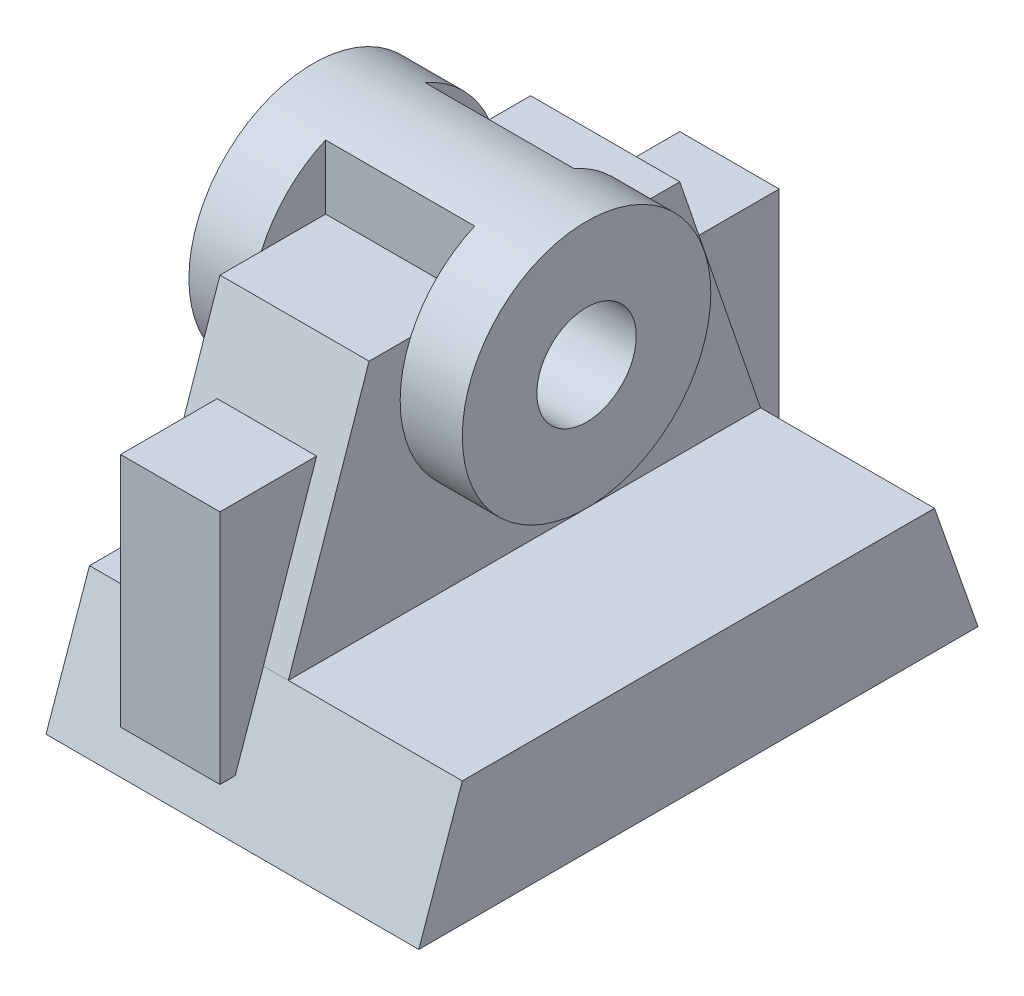
ISO-10303-21;
HEADER;
FILE_DESCRIPTION(('STEP AP214'),'2;1');
FILE_NAME('part.step','',(''),(''),'','','');
FILE_SCHEMA(('AUTOMOTIVE_DESIGN { 1 0 10303 214 1 1 1 1 }'));
ENDSEC;
DATA;
#1=APPLICATION_CONTEXT('core data for automotive mechanical design processes');
#2=APPLICATION_PROTOCOL_DEFINITION('international standard','automotive_design',2000,#1);
#3=PRODUCT_CONTEXT('',#1,'mechanical');
#4=PRODUCT('Part','Part','',(#3));
#5=PRODUCT_RELATED_PRODUCT_CATEGORY('part','',(#4));
#6=PRODUCT_DEFINITION_FORMATION('','',#4);
#7=PRODUCT_DEFINITION_CONTEXT('part definition',#1,'design');
#8=PRODUCT_DEFINITION('design','',#6,#7);
#9=PRODUCT_DEFINITION_SHAPE('','',#8);
#10=(LENGTH_UNIT() NAMED_UNIT(*) SI_UNIT(.MILLI.,.METRE.));
#11=(NAMED_UNIT(*) PLANE_ANGLE_UNIT() SI_UNIT($,.RADIAN.));
#12=(NAMED_UNIT(*) SI_UNIT($,.STERADIAN.) SOLID_ANGLE_UNIT());
#13=UNCERTAINTY_MEASURE_WITH_UNIT(LENGTH_MEASURE(1.E-05),#10,'distance_accuracy_value','');
#14=(GEOMETRIC_REPRESENTATION_CONTEXT(3) GLOBAL_UNCERTAINTY_ASSIGNED_CONTEXT((#13)) GLOBAL_UNIT_ASSIGNED_CONTEXT((#10,
#11,#12)) REPRESENTATION_CONTEXT('',''));
#15=CARTESIAN_POINT('',(0.,0.,0.));
#16=DIRECTION('',(0.,0.,1.));
#17=DIRECTION('',(1.,0.,0.));
#18=AXIS2_PLACEMENT_3D('',#15,#16,#17);
#19=CARTESIAN_POINT('',(-45.,20.,-38.));
#20=DIRECTION('',(0.,-0.330350424728106,0.943858356366018));
#21=DIRECTION('',(0.,-0.943858356366018,-0.330350424728106));
#22=AXIS2_PLACEMENT_3D('',#19,#20,#21);
#23=PLANE('',#22);
#24=DIRECTION('',(0.,-0.943858356366018,-0.330350424728106));
#25=VECTOR('',#24,1.);
#26=CARTESIAN_POINT('',(-2.,20.,-38.));
#27=LINE('',#26,#25);
#28=CARTESIAN_POINT('',(-2.,20.,-38.));
#29=VERTEX_POINT('',#28);
#30=CARTESIAN_POINT('',(-2.,7.,-42.55));
#31=VERTEX_POINT('',#30);
#32=EDGE_CURVE('E233',#29,#31,#27,.T.);
#33=ORIENTED_EDGE('',*,*,#32,.F.);
#34=DIRECTION('',(1.,0.,0.));
#35=VECTOR('',#34,1.);
#36=CARTESIAN_POINT('',(-22.,20.,-38.));
#37=LINE('',#36,#35);
#38=CARTESIAN_POINT('',(2.,20.,-38.));
#39=VERTEX_POINT('',#38);
#40=EDGE_CURVE('E332',#29,#39,#37,.T.);
#41=ORIENTED_EDGE('',*,*,#40,.T.);
#42=DIRECTION('',(1.,0.,0.));
#43=VECTOR('',#42,1.);
#44=CARTESIAN_POINT('',(-45.,20.,-38.));
#45=LINE('',#44,#43);
#46=CARTESIAN_POINT('',(30.,20.,-38.));
#47=VERTEX_POINT('',#46);
#48=EDGE_CURVE('E365',#39,#47,#45,.T.);
#49=ORIENTED_EDGE('',*,*,#48,.T.);
#50=DIRECTION('',(0.,-0.943858356366017,-0.330350424728106));
#51=VECTOR('',#50,1.);
#52=CARTESIAN_POINT('',(30.,20.,-38.));
#53=LINE('',#52,#51);
#54=CARTESIAN_POINT('',(30.,0.,-45.));
#55=VERTEX_POINT('',#54);
#56=EDGE_CURVE('E359',#47,#55,#53,.T.);
#57=ORIENTED_EDGE('',*,*,#56,.T.);
#58=DIRECTION('',(-1.,0.,0.));
#59=VECTOR('',#58,1.);
#60=CARTESIAN_POINT('',(30.,0.,-45.));
#61=LINE('',#60,#59);
#62=CARTESIAN_POINT('',(-30.,0.,-45.));
#63=VERTEX_POINT('',#62);
#64=EDGE_CURVE('E388',#55,#63,#61,.T.);
#65=ORIENTED_EDGE('',*,*,#64,.T.);
#66=DIRECTION('',(0.,-0.943858356366018,-0.330350424728106));
#67=VECTOR('',#66,1.);
#68=CARTESIAN_POINT('',(-30.,17.8173719376392,-38.7639198218263));
#69=LINE('',#68,#67);
#70=CARTESIAN_POINT('',(-30.,20.,-38.));
#71=VERTEX_POINT('',#70);
#72=EDGE_CURVE('E374',#71,#63,#69,.T.);
#73=ORIENTED_EDGE('',*,*,#72,.F.);
#74=CARTESIAN_POINT('',(-22.,20.,-38.));
#75=VERTEX_POINT('',#74);
#76=EDGE_CURVE('E364',#71,#75,#45,.T.);
#77=ORIENTED_EDGE('',*,*,#76,.T.);
#78=CARTESIAN_POINT('',(-18.,20.,-38.));
#79=VERTEX_POINT('',#78);
#80=EDGE_CURVE('E357',#75,#79,#37,.T.);
#81=ORIENTED_EDGE('',*,*,#80,.T.);
#82=DIRECTION('',(0.,0.943858356366018,0.330350424728106));
#83=VECTOR('',#82,1.);
#84=CARTESIAN_POINT('',(-18.,20.,-38.));
#85=LINE('',#84,#83);
#86=CARTESIAN_POINT('',(-18.,7.,-42.55));
#87=VERTEX_POINT('',#86);
#88=EDGE_CURVE('E53',#87,#79,#85,.T.);
#89=ORIENTED_EDGE('',*,*,#88,.F.);
#90=DIRECTION('',(-1.,0.,0.));
#91=VECTOR('',#90,1.);
#92=CARTESIAN_POINT('',(-45.,7.,-42.55));
#93=LINE('',#92,#91);
#94=EDGE_CURVE('E11',#31,#87,#93,.T.);
#95=ORIENTED_EDGE('',*,*,#94,.F.);
#96=EDGE_LOOP('',(#33,#41,#49,#57,#65,#73,#77,#81,#89,#95));
#97=FACE_BOUND('',#96,.T.);
#98=ADVANCED_FACE('F39',(#97),#23,.F.);
#99=CARTESIAN_POINT('',(-22.,20.,-38.));
#100=DIRECTION('',(0.,0.32368767906299,-0.946163984953356));
#101=DIRECTION('',(0.,0.946163984953356,0.32368767906299));
#102=AXIS2_PLACEMENT_3D('',#99,#100,#101);
#103=PLANE('',#102);
#104=ORIENTED_EDGE('',*,*,#40,.F.);
#105=DIRECTION('',(0.,0.946163984953356,0.32368767906299));
#106=VECTOR('',#105,1.);
#107=CARTESIAN_POINT('',(-2.,20.,-38.));
#108=LINE('',#107,#106);
#109=CARTESIAN_POINT('',(-2.,45.,-29.4473684210526));
#110=VERTEX_POINT('',#109);
#111=EDGE_CURVE('E50',#29,#110,#108,.T.);
#112=ORIENTED_EDGE('',*,*,#111,.T.);
#113=DIRECTION('',(-1.,0.,0.));
#114=VECTOR('',#113,1.);
#115=CARTESIAN_POINT('',(-22.,45.,-29.4473684210526));
#116=LINE('',#115,#114);
#117=CARTESIAN_POINT('',(-18.,45.,-29.4473684210526));
#118=VERTEX_POINT('',#117);
#119=EDGE_CURVE('E409',#110,#118,#116,.T.);
#120=ORIENTED_EDGE('',*,*,#119,.T.);
#121=DIRECTION('',(0.,-0.946163984953356,-0.32368767906299));
#122=VECTOR('',#121,1.);
#123=CARTESIAN_POINT('',(-18.,20.,-38.));
#124=LINE('',#123,#122);
#125=EDGE_CURVE('E404',#118,#79,#124,.T.);
#126=ORIENTED_EDGE('',*,*,#125,.T.);
#127=ORIENTED_EDGE('',*,*,#80,.F.);
#128=DIRECTION('',(0.,0.946163984953356,0.32368767906299));
#129=VECTOR('',#128,1.);
#130=CARTESIAN_POINT('',(-22.,20.,-38.));
#131=LINE('',#130,#129);
#132=CARTESIAN_POINT('',(-22.,58.,-25.));
#133=VERTEX_POINT('',#132);
#134=EDGE_CURVE('E314',#75,#133,#131,.T.);
#135=ORIENTED_EDGE('',*,*,#134,.T.);
#136=DIRECTION('',(1.,0.,0.));
#137=VECTOR('',#136,1.);
#138=CARTESIAN_POINT('',(-22.,58.,-25.));
#139=LINE('',#138,#137);
#140=CARTESIAN_POINT('',(2.,58.,-25.));
#141=VERTEX_POINT('',#140);
#142=EDGE_CURVE('E353',#133,#141,#139,.T.);
#143=ORIENTED_EDGE('',*,*,#142,.T.);
#144=DIRECTION('',(0.,0.946163984953356,0.32368767906299));
#145=VECTOR('',#144,1.);
#146=CARTESIAN_POINT('',(2.,20.,-38.));
#147=LINE('',#146,#145);
#148=EDGE_CURVE('E331',#39,#141,#147,.T.);
#149=ORIENTED_EDGE('',*,*,#148,.F.);
#150=EDGE_LOOP('',(#104,#112,#120,#126,#127,#135,#143,#149));
#151=FACE_BOUND('',#150,.T.);
#152=ADVANCED_FACE('F411',(#151),#103,.T.);
#153=CARTESIAN_POINT('',(-32.,50.,0.));
#154=DIRECTION('',(1.,0.,0.));
#155=DIRECTION('',(0.,0.,-1.));
#156=AXIS2_PLACEMENT_3D('',#153,#154,#155);
#157=CYLINDRICAL_SURFACE('',#156,20.);
#158=CARTESIAN_POINT('',(12.,50.,0.));
#159=DIRECTION('',(1.,0.,0.));
#160=DIRECTION('',(0.,0.,-1.));
#161=AXIS2_PLACEMENT_3D('',#158,#159,#160);
#162=CIRCLE('',#161,20.);
#163=CARTESIAN_POINT('',(12.,50.,-20.));
#164=VERTEX_POINT('',#163);
#165=EDGE_CURVE('E302',#164,#164,#162,.T.);
#166=ORIENTED_EDGE('',*,*,#165,.F.);
#167=EDGE_LOOP('',(#166));
#168=FACE_BOUND('',#167,.T.);
#169=CARTESIAN_POINT('',(-32.,50.,0.));
#170=DIRECTION('',(1.,0.,0.));
#171=DIRECTION('',(0.,0.,-1.));
#172=AXIS2_PLACEMENT_3D('',#169,#170,#171);
#173=CIRCLE('',#172,20.);
#174=CARTESIAN_POINT('',(-32.,50.,-20.));
#175=VERTEX_POINT('',#174);
#176=EDGE_CURVE('E306',#175,#175,#173,.T.);
#177=ORIENTED_EDGE('',*,*,#176,.T.);
#178=EDGE_LOOP('',(#177));
#179=FACE_BOUND('',#178,.T.);
#180=DIRECTION('',(1.,0.,0.));
#181=VECTOR('',#180,1.);
#182=CARTESIAN_POINT('',(-22.,68.3303027798234,-8.));
#183=LINE('',#182,#181);
#184=CARTESIAN_POINT('',(-22.,68.3303027798234,-8.));
#185=VERTEX_POINT('',#184);
#186=CARTESIAN_POINT('',(2.,68.3303027798234,-8.));
#187=VERTEX_POINT('',#186);
#188=EDGE_CURVE('E275',#185,#187,#183,.T.);
#189=ORIENTED_EDGE('',*,*,#188,.F.);
#190=CARTESIAN_POINT('',(-22.,50.,0.));
#191=DIRECTION('',(-1.,0.,0.));
#192=DIRECTION('',(0.,0.,1.));
#193=AXIS2_PLACEMENT_3D('',#190,#191,#192);
#194=CIRCLE('',#193,20.);
#195=CARTESIAN_POINT('',(-22.,58.,-18.3303027798234));
#196=VERTEX_POINT('',#195);
#197=EDGE_CURVE('E262',#185,#196,#194,.T.);
#198=ORIENTED_EDGE('',*,*,#197,.T.);
#199=CARTESIAN_POINT('',(-22.,50.,0.));
#200=DIRECTION('',(-1.,0.,0.));
#201=DIRECTION('',(0.,0.,-1.));
#202=AXIS2_PLACEMENT_3D('',#199,#200,#201);
#203=CIRCLE('',#202,20.);
#204=CARTESIAN_POINT('',(-22.,58.,18.3303027798234));
#205=VERTEX_POINT('',#204);
#206=EDGE_CURVE('E321',#196,#205,#203,.T.);
#207=ORIENTED_EDGE('',*,*,#206,.T.);
#208=CARTESIAN_POINT('',(-22.,50.,0.));
#209=DIRECTION('',(1.,0.,0.));
#210=DIRECTION('',(0.,0.,-1.));
#211=AXIS2_PLACEMENT_3D('',#208,#209,#210);
#212=CIRCLE('',#211,20.);
#213=CARTESIAN_POINT('',(-22.,68.3303027798234,8.));
#214=VERTEX_POINT('',#213);
#215=EDGE_CURVE('E283',#214,#205,#212,.T.);
#216=ORIENTED_EDGE('',*,*,#215,.F.);
#217=DIRECTION('',(1.,0.,0.));
#218=VECTOR('',#217,1.);
#219=CARTESIAN_POINT('',(-22.,68.3303027798234,8.));
#220=LINE('',#219,#218);
#221=CARTESIAN_POINT('',(2.,68.3303027798234,8.));
#222=VERTEX_POINT('',#221);
#223=EDGE_CURVE('E301',#214,#222,#220,.T.);
#224=ORIENTED_EDGE('',*,*,#223,.T.);
#225=CARTESIAN_POINT('',(2.,50.,0.));
#226=DIRECTION('',(1.,0.,0.));
#227=DIRECTION('',(0.,0.,-1.));
#228=AXIS2_PLACEMENT_3D('',#225,#226,#227);
#229=CIRCLE('',#228,20.);
#230=CARTESIAN_POINT('',(2.,58.,18.3303027798234));
#231=VERTEX_POINT('',#230);
#232=EDGE_CURVE('E277',#222,#231,#229,.T.);
#233=ORIENTED_EDGE('',*,*,#232,.T.);
#234=CARTESIAN_POINT('',(2.,50.,0.));
#235=DIRECTION('',(-1.,0.,0.));
#236=DIRECTION('',(0.,0.,-1.));
#237=AXIS2_PLACEMENT_3D('',#234,#235,#236);
#238=CIRCLE('',#237,20.);
#239=CARTESIAN_POINT('',(2.,58.,-18.3303027798234));
#240=VERTEX_POINT('',#239);
#241=EDGE_CURVE('E338',#240,#231,#238,.T.);
#242=ORIENTED_EDGE('',*,*,#241,.F.);
#243=CARTESIAN_POINT('',(2.,50.,0.));
#244=DIRECTION('',(-1.,0.,0.));
#245=DIRECTION('',(0.,0.,1.));
#246=AXIS2_PLACEMENT_3D('',#243,#244,#245);
#247=CIRCLE('',#246,20.);
#248=EDGE_CURVE('E263',#187,#240,#247,.T.);
#249=ORIENTED_EDGE('',*,*,#248,.F.);
#250=EDGE_LOOP('',(#189,#198,#207,#216,#224,#233,#242,#249));
#251=FACE_BOUND('',#250,.T.);
#252=ADVANCED_FACE('F487',(#168,#179,#251),#157,.T.);
#253=CARTESIAN_POINT('',(0.,20.,0.));
#254=DIRECTION('',(0.,1.,0.));
#255=DIRECTION('',(0.,0.,1.));
#256=AXIS2_PLACEMENT_3D('',#253,#254,#255);
#257=PLANE('',#256);
#258=DIRECTION('',(1.,0.,0.));
#259=VECTOR('',#258,1.);
#260=CARTESIAN_POINT('',(-45.,20.,38.));
#261=LINE('',#260,#259);
#262=CARTESIAN_POINT('',(-30.,20.,38.));
#263=VERTEX_POINT('',#262);
#264=CARTESIAN_POINT('',(-22.,20.,38.));
#265=VERTEX_POINT('',#264);
#266=EDGE_CURVE('E361',#263,#265,#261,.T.);
#267=ORIENTED_EDGE('',*,*,#266,.T.);
#268=DIRECTION('',(0.,0.,-1.));
#269=VECTOR('',#268,1.);
#270=CARTESIAN_POINT('',(-22.,20.,38.));
#271=LINE('',#270,#269);
#272=EDGE_CURVE('E315',#265,#75,#271,.T.);
#273=ORIENTED_EDGE('',*,*,#272,.T.);
#274=ORIENTED_EDGE('',*,*,#76,.F.);
#275=DIRECTION('',(0.,0.,1.));
#276=VECTOR('',#275,1.);
#277=CARTESIAN_POINT('',(-30.,20.,-45.));
#278=LINE('',#277,#276);
#279=EDGE_CURVE('E385',#71,#263,#278,.T.);
#280=ORIENTED_EDGE('',*,*,#279,.T.);
#281=EDGE_LOOP('',(#267,#273,#274,#280));
#282=FACE_BOUND('',#281,.T.);
#283=ADVANCED_FACE('F423',(#282),#257,.T.);
#284=CARTESIAN_POINT('',(30.,20.,0.));
#285=DIRECTION('',(-1.,0.,0.));
#286=DIRECTION('',(0.,0.,1.));
#287=AXIS2_PLACEMENT_3D('',#284,#285,#286);
#288=PLANE('',#287);
#289=DIRECTION('',(0.,0.,-1.));
#290=VECTOR('',#289,1.);
#291=CARTESIAN_POINT('',(30.,0.,0.));
#292=LINE('',#291,#290);
#293=CARTESIAN_POINT('',(30.,0.,45.));
#294=VERTEX_POINT('',#293);
#295=EDGE_CURVE('E377',#294,#55,#292,.T.);
#296=ORIENTED_EDGE('',*,*,#295,.T.);
#297=ORIENTED_EDGE('',*,*,#56,.F.);
#298=DIRECTION('',(0.,0.,-1.));
#299=VECTOR('',#298,1.);
#300=CARTESIAN_POINT('',(30.,20.,45.));
#301=LINE('',#300,#299);
#302=CARTESIAN_POINT('',(30.,20.,38.));
#303=VERTEX_POINT('',#302);
#304=EDGE_CURVE('E378',#303,#47,#301,.T.);
#305=ORIENTED_EDGE('',*,*,#304,.F.);
#306=DIRECTION('',(0.,0.943858356366017,-0.330350424728106));
#307=VECTOR('',#306,1.);
#308=CARTESIAN_POINT('',(30.,20.,38.));
#309=LINE('',#308,#307);
#310=EDGE_CURVE('E352',#294,#303,#309,.T.);
#311=ORIENTED_EDGE('',*,*,#310,.F.);
#312=EDGE_LOOP('',(#296,#297,#305,#311));
#313=FACE_BOUND('',#312,.T.);
#314=ADVANCED_FACE('F41',(#313),#288,.F.);
#315=CARTESIAN_POINT('',(-30.,20.,-45.));
#316=DIRECTION('',(1.,0.,0.));
#317=DIRECTION('',(0.,0.,-1.));
#318=AXIS2_PLACEMENT_3D('',#315,#316,#317);
#319=PLANE('',#318);
#320=ORIENTED_EDGE('',*,*,#279,.F.);
#321=ORIENTED_EDGE('',*,*,#72,.T.);
#322=DIRECTION('',(0.,0.,1.));
#323=VECTOR('',#322,1.);
#324=CARTESIAN_POINT('',(-30.,0.,-45.));
#325=LINE('',#324,#323);
#326=CARTESIAN_POINT('',(-30.,0.,45.));
#327=VERTEX_POINT('',#326);
#328=EDGE_CURVE('E391',#63,#327,#325,.T.);
#329=ORIENTED_EDGE('',*,*,#328,.T.);
#330=DIRECTION('',(0.,0.943858356366017,-0.330350424728106));
#331=VECTOR('',#330,1.);
#332=CARTESIAN_POINT('',(-30.,45.8797327394209,28.9420935412027));
#333=LINE('',#332,#331);
#334=EDGE_CURVE('E370',#327,#263,#333,.T.);
#335=ORIENTED_EDGE('',*,*,#334,.T.);
#336=EDGE_LOOP('',(#320,#321,#329,#335));
#337=FACE_BOUND('',#336,.T.);
#338=ADVANCED_FACE('F471',(#337),#319,.F.);
#339=DIRECTION('',(0.,0.,-1.));
#340=VECTOR('',#339,1.);
#341=CARTESIAN_POINT('',(2.,20.,-38.));
#342=LINE('',#341,#340);
#343=CARTESIAN_POINT('',(2.,20.,38.));
#344=VERTEX_POINT('',#343);
#345=EDGE_CURVE('E307',#344,#39,#342,.T.);
#346=ORIENTED_EDGE('',*,*,#345,.F.);
#347=EDGE_CURVE('E369',#344,#303,#261,.T.);
#348=ORIENTED_EDGE('',*,*,#347,.T.);
#349=ORIENTED_EDGE('',*,*,#304,.T.);
#350=ORIENTED_EDGE('',*,*,#48,.F.);
#351=EDGE_LOOP('',(#346,#348,#349,#350));
#352=FACE_BOUND('',#351,.T.);
#353=ADVANCED_FACE('F459',(#352),#257,.T.);
#354=CARTESIAN_POINT('',(0.,0.,0.));
#355=DIRECTION('',(0.,1.,0.));
#356=DIRECTION('',(0.,0.,1.));
#357=AXIS2_PLACEMENT_3D('',#354,#355,#356);
#358=PLANE('',#357);
#359=ORIENTED_EDGE('',*,*,#295,.F.);
#360=DIRECTION('',(1.,0.,0.));
#361=VECTOR('',#360,1.);
#362=CARTESIAN_POINT('',(-30.,0.,45.));
#363=LINE('',#362,#361);
#364=EDGE_CURVE('E384',#327,#294,#363,.T.);
#365=ORIENTED_EDGE('',*,*,#364,.F.);
#366=ORIENTED_EDGE('',*,*,#328,.F.);
#367=ORIENTED_EDGE('',*,*,#64,.F.);
#368=EDGE_LOOP('',(#359,#365,#366,#367));
#369=FACE_BOUND('',#368,.T.);
#370=ADVANCED_FACE('F468',(#369),#358,.F.);
#371=CARTESIAN_POINT('',(-45.,20.,38.));
#372=DIRECTION('',(0.,-0.330350424728106,-0.943858356366017));
#373=DIRECTION('',(0.,0.943858356366017,-0.330350424728106));
#374=AXIS2_PLACEMENT_3D('',#371,#372,#373);
#375=PLANE('',#374);
#376=DIRECTION('',(-1.,0.,0.));
#377=VECTOR('',#376,1.);
#378=CARTESIAN_POINT('',(-45.,7.,42.55));
#379=LINE('',#378,#377);
#380=CARTESIAN_POINT('',(-2.,7.,42.55));
#381=VERTEX_POINT('',#380);
#382=CARTESIAN_POINT('',(-18.,7.,42.55));
#383=VERTEX_POINT('',#382);
#384=EDGE_CURVE('E61',#381,#383,#379,.T.);
#385=ORIENTED_EDGE('',*,*,#384,.T.);
#386=DIRECTION('',(0.,0.943858356366017,-0.330350424728106));
#387=VECTOR('',#386,1.);
#388=CARTESIAN_POINT('',(-18.,20.,38.));
#389=LINE('',#388,#387);
#390=CARTESIAN_POINT('',(-18.,20.,38.));
#391=VERTEX_POINT('',#390);
#392=EDGE_CURVE('E253',#383,#391,#389,.T.);
#393=ORIENTED_EDGE('',*,*,#392,.T.);
#394=DIRECTION('',(1.,0.,0.));
#395=VECTOR('',#394,1.);
#396=CARTESIAN_POINT('',(-22.,20.,38.));
#397=LINE('',#396,#395);
#398=EDGE_CURVE('E348',#265,#391,#397,.T.);
#399=ORIENTED_EDGE('',*,*,#398,.F.);
#400=ORIENTED_EDGE('',*,*,#266,.F.);
#401=ORIENTED_EDGE('',*,*,#334,.F.);
#402=ORIENTED_EDGE('',*,*,#364,.T.);
#403=ORIENTED_EDGE('',*,*,#310,.T.);
#404=ORIENTED_EDGE('',*,*,#347,.F.);
#405=CARTESIAN_POINT('',(-2.,20.,38.));
#406=VERTEX_POINT('',#405);
#407=EDGE_CURVE('E355',#406,#344,#397,.T.);
#408=ORIENTED_EDGE('',*,*,#407,.F.);
#409=DIRECTION('',(0.,-0.943858356366017,0.330350424728106));
#410=VECTOR('',#409,1.);
#411=CARTESIAN_POINT('',(-2.,20.,38.));
#412=LINE('',#411,#410);
#413=EDGE_CURVE('E247',#406,#381,#412,.T.);
#414=ORIENTED_EDGE('',*,*,#413,.T.);
#415=EDGE_LOOP('',(#385,#393,#399,#400,#401,#402,#403,#404,#408,#414));
#416=FACE_BOUND('',#415,.T.);
#417=ADVANCED_FACE('F435',(#416),#375,.F.);
#418=CARTESIAN_POINT('',(-22.,20.,38.));
#419=DIRECTION('',(0.,0.32368767906299,0.946163984953356));
#420=DIRECTION('',(0.,-0.946163984953356,0.32368767906299));
#421=AXIS2_PLACEMENT_3D('',#418,#419,#420);
#422=PLANE('',#421);
#423=DIRECTION('',(0.,-0.946163984953356,0.32368767906299));
#424=VECTOR('',#423,1.);
#425=CARTESIAN_POINT('',(-18.,20.,38.));
#426=LINE('',#425,#424);
#427=CARTESIAN_POINT('',(-18.,45.,29.4473684210526));
#428=VERTEX_POINT('',#427);
#429=EDGE_CURVE('E398',#428,#391,#426,.T.);
#430=ORIENTED_EDGE('',*,*,#429,.F.);
#431=DIRECTION('',(-1.,0.,0.));
#432=VECTOR('',#431,1.);
#433=CARTESIAN_POINT('',(-22.,45.,29.4473684210526));
#434=LINE('',#433,#432);
#435=CARTESIAN_POINT('',(-2.,45.,29.4473684210526));
#436=VERTEX_POINT('',#435);
#437=EDGE_CURVE('E400',#436,#428,#434,.T.);
#438=ORIENTED_EDGE('',*,*,#437,.F.);
#439=DIRECTION('',(0.,0.946163984953356,-0.32368767906299));
#440=VECTOR('',#439,1.);
#441=CARTESIAN_POINT('',(-2.,20.,38.));
#442=LINE('',#441,#440);
#443=EDGE_CURVE('E389',#406,#436,#442,.T.);
#444=ORIENTED_EDGE('',*,*,#443,.F.);
#445=ORIENTED_EDGE('',*,*,#407,.T.);
#446=DIRECTION('',(0.,-0.946163984953356,0.32368767906299));
#447=VECTOR('',#446,1.);
#448=CARTESIAN_POINT('',(2.,20.,38.));
#449=LINE('',#448,#447);
#450=CARTESIAN_POINT('',(2.,58.,25.));
#451=VERTEX_POINT('',#450);
#452=EDGE_CURVE('E317',#451,#344,#449,.T.);
#453=ORIENTED_EDGE('',*,*,#452,.F.);
#454=DIRECTION('',(1.,0.,0.));
#455=VECTOR('',#454,1.);
#456=CARTESIAN_POINT('',(-22.,58.,25.));
#457=LINE('',#456,#455);
#458=CARTESIAN_POINT('',(-22.,58.,25.));
#459=VERTEX_POINT('',#458);
#460=EDGE_CURVE('E354',#459,#451,#457,.T.);
#461=ORIENTED_EDGE('',*,*,#460,.F.);
#462=DIRECTION('',(0.,-0.946163984953356,0.32368767906299));
#463=VECTOR('',#462,1.);
#464=CARTESIAN_POINT('',(-22.,20.,38.));
#465=LINE('',#464,#463);
#466=EDGE_CURVE('E328',#459,#265,#465,.T.);
#467=ORIENTED_EDGE('',*,*,#466,.T.);
#468=ORIENTED_EDGE('',*,*,#398,.T.);
#469=EDGE_LOOP('',(#430,#438,#444,#445,#453,#461,#467,#468));
#470=FACE_BOUND('',#469,.T.);
#471=ADVANCED_FACE('F427',(#470),#422,.T.);
#472=CARTESIAN_POINT('',(-22.,58.,25.));
#473=DIRECTION('',(0.,1.,0.));
#474=DIRECTION('',(0.,0.,1.));
#475=AXIS2_PLACEMENT_3D('',#472,#473,#474);
#476=PLANE('',#475);
#477=DIRECTION('',(0.,0.,1.));
#478=VECTOR('',#477,1.);
#479=CARTESIAN_POINT('',(2.,58.,25.));
#480=LINE('',#479,#478);
#481=EDGE_CURVE('E345',#231,#451,#480,.T.);
#482=ORIENTED_EDGE('',*,*,#481,.F.);
#483=DIRECTION('',(0.,0.,-1.));
#484=VECTOR('',#483,1.);
#485=CARTESIAN_POINT('',(2.,58.,18.3303027798234));
#486=LINE('',#485,#484);
#487=CARTESIAN_POINT('',(2.,58.,8.));
#488=VERTEX_POINT('',#487);
#489=EDGE_CURVE('E298',#231,#488,#486,.T.);
#490=ORIENTED_EDGE('',*,*,#489,.T.);
#491=DIRECTION('',(1.,0.,0.));
#492=VECTOR('',#491,1.);
#493=CARTESIAN_POINT('',(-22.,58.,8.));
#494=LINE('',#493,#492);
#495=CARTESIAN_POINT('',(-22.,58.,8.));
#496=VERTEX_POINT('',#495);
#497=EDGE_CURVE('E291',#496,#488,#494,.T.);
#498=ORIENTED_EDGE('',*,*,#497,.F.);
#499=DIRECTION('',(0.,0.,-1.));
#500=VECTOR('',#499,1.);
#501=CARTESIAN_POINT('',(-22.,58.,18.3303027798234));
#502=LINE('',#501,#500);
#503=EDGE_CURVE('E287',#205,#496,#502,.T.);
#504=ORIENTED_EDGE('',*,*,#503,.F.);
#505=DIRECTION('',(0.,0.,1.));
#506=VECTOR('',#505,1.);
#507=CARTESIAN_POINT('',(-22.,58.,25.));
#508=LINE('',#507,#506);
#509=EDGE_CURVE('E322',#205,#459,#508,.T.);
#510=ORIENTED_EDGE('',*,*,#509,.T.);
#511=ORIENTED_EDGE('',*,*,#460,.T.);
#512=EDGE_LOOP('',(#482,#490,#498,#504,#510,#511));
#513=FACE_BOUND('',#512,.T.);
#514=ADVANCED_FACE('F512',(#513),#476,.T.);
#515=CARTESIAN_POINT('',(-22.,58.,-25.));
#516=DIRECTION('',(0.,1.,0.));
#517=DIRECTION('',(0.,0.,1.));
#518=AXIS2_PLACEMENT_3D('',#515,#516,#517);
#519=PLANE('',#518);
#520=DIRECTION('',(0.,0.,1.));
#521=VECTOR('',#520,1.);
#522=CARTESIAN_POINT('',(2.,58.,-25.));
#523=LINE('',#522,#521);
#524=EDGE_CURVE('E340',#141,#240,#523,.T.);
#525=ORIENTED_EDGE('',*,*,#524,.F.);
#526=ORIENTED_EDGE('',*,*,#142,.F.);
#527=DIRECTION('',(0.,0.,1.));
#528=VECTOR('',#527,1.);
#529=CARTESIAN_POINT('',(-22.,58.,-25.));
#530=LINE('',#529,#528);
#531=EDGE_CURVE('E316',#133,#196,#530,.T.);
#532=ORIENTED_EDGE('',*,*,#531,.T.);
#533=DIRECTION('',(0.,0.,1.));
#534=VECTOR('',#533,1.);
#535=CARTESIAN_POINT('',(-22.,58.,-18.3303027798234));
#536=LINE('',#535,#534);
#537=CARTESIAN_POINT('',(-22.,58.,-8.));
#538=VERTEX_POINT('',#537);
#539=EDGE_CURVE('E268',#196,#538,#536,.T.);
#540=ORIENTED_EDGE('',*,*,#539,.T.);
#541=DIRECTION('',(1.,0.,0.));
#542=VECTOR('',#541,1.);
#543=CARTESIAN_POINT('',(-22.,58.,-8.));
#544=LINE('',#543,#542);
#545=CARTESIAN_POINT('',(2.,58.,-8.));
#546=VERTEX_POINT('',#545);
#547=EDGE_CURVE('E276',#538,#546,#544,.T.);
#548=ORIENTED_EDGE('',*,*,#547,.T.);
#549=DIRECTION('',(0.,0.,1.));
#550=VECTOR('',#549,1.);
#551=CARTESIAN_POINT('',(2.,58.,-18.3303027798234));
#552=LINE('',#551,#550);
#553=EDGE_CURVE('E269',#240,#546,#552,.T.);
#554=ORIENTED_EDGE('',*,*,#553,.F.);
#555=EDGE_LOOP('',(#525,#526,#532,#540,#548,#554));
#556=FACE_BOUND('',#555,.T.);
#557=ADVANCED_FACE('F513',(#556),#519,.T.);
#558=CARTESIAN_POINT('',(-22.,50.,0.));
#559=DIRECTION('',(1.,0.,0.));
#560=DIRECTION('',(0.,0.,-1.));
#561=AXIS2_PLACEMENT_3D('',#558,#559,#560);
#562=PLANE('',#561);
#563=ORIENTED_EDGE('',*,*,#272,.F.);
#564=ORIENTED_EDGE('',*,*,#466,.F.);
#565=ORIENTED_EDGE('',*,*,#509,.F.);
#566=ORIENTED_EDGE('',*,*,#206,.F.);
#567=ORIENTED_EDGE('',*,*,#531,.F.);
#568=ORIENTED_EDGE('',*,*,#134,.F.);
#569=EDGE_LOOP('',(#563,#564,#565,#566,#567,#568));
#570=FACE_BOUND('',#569,.T.);
#571=ADVANCED_FACE('F424',(#570),#562,.F.);
#572=CARTESIAN_POINT('',(2.,50.,0.));
#573=DIRECTION('',(1.,0.,0.));
#574=DIRECTION('',(0.,0.,-1.));
#575=AXIS2_PLACEMENT_3D('',#572,#573,#574);
#576=PLANE('',#575);
#577=ORIENTED_EDGE('',*,*,#452,.T.);
#578=ORIENTED_EDGE('',*,*,#345,.T.);
#579=ORIENTED_EDGE('',*,*,#148,.T.);
#580=ORIENTED_EDGE('',*,*,#524,.T.);
#581=ORIENTED_EDGE('',*,*,#241,.T.);
#582=ORIENTED_EDGE('',*,*,#481,.T.);
#583=EDGE_LOOP('',(#577,#578,#579,#580,#581,#582));
#584=FACE_BOUND('',#583,.T.);
#585=ADVANCED_FACE('F456',(#584),#576,.T.);
#586=CARTESIAN_POINT('',(-32.,50.,0.));
#587=DIRECTION('',(1.,0.,0.));
#588=DIRECTION('',(0.,0.,-1.));
#589=AXIS2_PLACEMENT_3D('',#586,#587,#588);
#590=PLANE('',#589);
#591=CARTESIAN_POINT('',(-32.,50.,0.));
#592=DIRECTION('',(1.,0.,0.));
#593=DIRECTION('',(0.,0.,-1.));
#594=AXIS2_PLACEMENT_3D('',#591,#592,#593);
#595=CIRCLE('',#594,8.);
#596=CARTESIAN_POINT('',(-32.,50.,-8.));
#597=VERTEX_POINT('',#596);
#598=EDGE_CURVE('E257',#597,#597,#595,.T.);
#599=ORIENTED_EDGE('',*,*,#598,.T.);
#600=EDGE_LOOP('',(#599));
#601=FACE_BOUND('',#600,.T.);
#602=ORIENTED_EDGE('',*,*,#176,.F.);
#603=EDGE_LOOP('',(#602));
#604=FACE_BOUND('',#603,.T.);
#605=ADVANCED_FACE('F577',(#601,#604),#590,.F.);
#606=CARTESIAN_POINT('',(12.,50.,0.));
#607=DIRECTION('',(1.,0.,0.));
#608=DIRECTION('',(0.,0.,-1.));
#609=AXIS2_PLACEMENT_3D('',#606,#607,#608);
#610=PLANE('',#609);
#611=CARTESIAN_POINT('',(12.,50.,0.));
#612=DIRECTION('',(1.,0.,0.));
#613=DIRECTION('',(0.,0.,-1.));
#614=AXIS2_PLACEMENT_3D('',#611,#612,#613);
#615=CIRCLE('',#614,8.);
#616=CARTESIAN_POINT('',(12.,50.,-8.));
#617=VERTEX_POINT('',#616);
#618=EDGE_CURVE('E256',#617,#617,#615,.T.);
#619=ORIENTED_EDGE('',*,*,#618,.F.);
#620=EDGE_LOOP('',(#619));
#621=FACE_BOUND('',#620,.T.);
#622=ORIENTED_EDGE('',*,*,#165,.T.);
#623=EDGE_LOOP('',(#622));
#624=FACE_BOUND('',#623,.T.);
#625=ADVANCED_FACE('F530',(#621,#624),#610,.T.);
#626=CARTESIAN_POINT('',(-22.,68.3303027798234,8.));
#627=DIRECTION('',(0.,0.,-1.));
#628=DIRECTION('',(-1.,0.,0.));
#629=AXIS2_PLACEMENT_3D('',#626,#627,#628);
#630=PLANE('',#629);
#631=DIRECTION('',(0.,1.,0.));
#632=VECTOR('',#631,1.);
#633=CARTESIAN_POINT('',(2.,68.3303027798234,8.));
#634=LINE('',#633,#632);
#635=EDGE_CURVE('E290',#488,#222,#634,.T.);
#636=ORIENTED_EDGE('',*,*,#635,.T.);
#637=ORIENTED_EDGE('',*,*,#223,.F.);
#638=DIRECTION('',(0.,1.,0.));
#639=VECTOR('',#638,1.);
#640=CARTESIAN_POINT('',(-22.,68.3303027798234,8.));
#641=LINE('',#640,#639);
#642=EDGE_CURVE('E288',#496,#214,#641,.T.);
#643=ORIENTED_EDGE('',*,*,#642,.F.);
#644=ORIENTED_EDGE('',*,*,#497,.T.);
#645=EDGE_LOOP('',(#636,#637,#643,#644));
#646=FACE_BOUND('',#645,.T.);
#647=ADVANCED_FACE('F523',(#646),#630,.F.);
#648=CARTESIAN_POINT('',(-22.,50.,0.));
#649=DIRECTION('',(1.,0.,0.));
#650=DIRECTION('',(0.,0.,-1.));
#651=AXIS2_PLACEMENT_3D('',#648,#649,#650);
#652=PLANE('',#651);
#653=ORIENTED_EDGE('',*,*,#215,.T.);
#654=ORIENTED_EDGE('',*,*,#503,.T.);
#655=ORIENTED_EDGE('',*,*,#642,.T.);
#656=EDGE_LOOP('',(#653,#654,#655));
#657=FACE_BOUND('',#656,.T.);
#658=ADVANCED_FACE('F527',(#657),#652,.T.);
#659=CARTESIAN_POINT('',(2.,50.,0.));
#660=DIRECTION('',(1.,0.,0.));
#661=DIRECTION('',(0.,0.,-1.));
#662=AXIS2_PLACEMENT_3D('',#659,#660,#661);
#663=PLANE('',#662);
#664=ORIENTED_EDGE('',*,*,#232,.F.);
#665=ORIENTED_EDGE('',*,*,#635,.F.);
#666=ORIENTED_EDGE('',*,*,#489,.F.);
#667=EDGE_LOOP('',(#664,#665,#666));
#668=FACE_BOUND('',#667,.T.);
#669=ADVANCED_FACE('F539',(#668),#663,.F.);
#670=CARTESIAN_POINT('',(-22.,68.3303027798234,-8.));
#671=DIRECTION('',(0.,0.,-1.));
#672=DIRECTION('',(-1.,0.,0.));
#673=AXIS2_PLACEMENT_3D('',#670,#671,#672);
#674=PLANE('',#673);
#675=DIRECTION('',(0.,1.,0.));
#676=VECTOR('',#675,1.);
#677=CARTESIAN_POINT('',(2.,68.3303027798234,-8.));
#678=LINE('',#677,#676);
#679=EDGE_CURVE('E274',#546,#187,#678,.T.);
#680=ORIENTED_EDGE('',*,*,#679,.F.);
#681=ORIENTED_EDGE('',*,*,#547,.F.);
#682=DIRECTION('',(0.,1.,0.));
#683=VECTOR('',#682,1.);
#684=CARTESIAN_POINT('',(-22.,68.3303027798234,-8.));
#685=LINE('',#684,#683);
#686=EDGE_CURVE('E270',#538,#185,#685,.T.);
#687=ORIENTED_EDGE('',*,*,#686,.T.);
#688=ORIENTED_EDGE('',*,*,#188,.T.);
#689=EDGE_LOOP('',(#680,#681,#687,#688));
#690=FACE_BOUND('',#689,.T.);
#691=ADVANCED_FACE('F544',(#690),#674,.T.);
#692=CARTESIAN_POINT('',(-22.,50.,0.));
#693=DIRECTION('',(1.,0.,0.));
#694=DIRECTION('',(0.,0.,1.));
#695=AXIS2_PLACEMENT_3D('',#692,#693,#694);
#696=PLANE('',#695);
#697=ORIENTED_EDGE('',*,*,#197,.F.);
#698=ORIENTED_EDGE('',*,*,#686,.F.);
#699=ORIENTED_EDGE('',*,*,#539,.F.);
#700=EDGE_LOOP('',(#697,#698,#699));
#701=FACE_BOUND('',#700,.T.);
#702=ADVANCED_FACE('F585',(#701),#696,.T.);
#703=CARTESIAN_POINT('',(2.,50.,0.));
#704=DIRECTION('',(1.,0.,0.));
#705=DIRECTION('',(0.,0.,1.));
#706=AXIS2_PLACEMENT_3D('',#703,#704,#705);
#707=PLANE('',#706);
#708=ORIENTED_EDGE('',*,*,#248,.T.);
#709=ORIENTED_EDGE('',*,*,#553,.T.);
#710=ORIENTED_EDGE('',*,*,#679,.T.);
#711=EDGE_LOOP('',(#708,#709,#710));
#712=FACE_BOUND('',#711,.T.);
#713=ADVANCED_FACE('F595',(#712),#707,.F.);
#714=CARTESIAN_POINT('',(-45.,50.,0.));
#715=DIRECTION('',(1.,0.,0.));
#716=DIRECTION('',(0.,0.,-1.));
#717=AXIS2_PLACEMENT_3D('',#714,#715,#716);
#718=CYLINDRICAL_SURFACE('',#717,8.);
#719=ORIENTED_EDGE('',*,*,#618,.T.);
#720=EDGE_LOOP('',(#719));
#721=FACE_BOUND('',#720,.T.);
#722=ORIENTED_EDGE('',*,*,#598,.F.);
#723=EDGE_LOOP('',(#722));
#724=FACE_BOUND('',#723,.T.);
#725=ADVANCED_FACE('F604',(#721,#724),#718,.F.);
#726=CARTESIAN_POINT('',(-10.,7.,25.));
#727=DIRECTION('',(0.,-1.,0.));
#728=DIRECTION('',(0.,0.,-1.));
#729=AXIS2_PLACEMENT_3D('',#726,#727,#728);
#730=PLANE('',#729);
#731=ORIENTED_EDGE('',*,*,#384,.F.);
#732=DIRECTION('',(0.,0.,1.));
#733=VECTOR('',#732,1.);
#734=CARTESIAN_POINT('',(-2.,7.,25.));
#735=LINE('',#734,#733);
#736=CARTESIAN_POINT('',(-2.,7.,45.));
#737=VERTEX_POINT('',#736);
#738=EDGE_CURVE('E244',#381,#737,#735,.T.);
#739=ORIENTED_EDGE('',*,*,#738,.T.);
#740=DIRECTION('',(1.,0.,0.));
#741=VECTOR('',#740,1.);
#742=CARTESIAN_POINT('',(-10.,7.,45.));
#743=LINE('',#742,#741);
#744=CARTESIAN_POINT('',(-18.,7.,45.));
#745=VERTEX_POINT('',#744);
#746=EDGE_CURVE('E231',#745,#737,#743,.T.);
#747=ORIENTED_EDGE('',*,*,#746,.F.);
#748=DIRECTION('',(0.,0.,1.));
#749=VECTOR('',#748,1.);
#750=CARTESIAN_POINT('',(-18.,7.,25.));
#751=LINE('',#750,#749);
#752=EDGE_CURVE('E246',#383,#745,#751,.T.);
#753=ORIENTED_EDGE('',*,*,#752,.F.);
#754=EDGE_LOOP('',(#731,#739,#747,#753));
#755=FACE_BOUND('',#754,.T.);
#756=ADVANCED_FACE('F439',(#755),#730,.T.);
#757=CARTESIAN_POINT('',(-18.,45.,25.));
#758=DIRECTION('',(-1.,0.,0.));
#759=DIRECTION('',(0.,0.,1.));
#760=AXIS2_PLACEMENT_3D('',#757,#758,#759);
#761=PLANE('',#760);
#762=ORIENTED_EDGE('',*,*,#392,.F.);
#763=ORIENTED_EDGE('',*,*,#752,.T.);
#764=DIRECTION('',(0.,-1.,0.));
#765=VECTOR('',#764,1.);
#766=CARTESIAN_POINT('',(-18.,45.,45.));
#767=LINE('',#766,#765);
#768=CARTESIAN_POINT('',(-18.,45.,45.));
#769=VERTEX_POINT('',#768);
#770=EDGE_CURVE('E245',#769,#745,#767,.T.);
#771=ORIENTED_EDGE('',*,*,#770,.F.);
#772=DIRECTION('',(0.,0.,1.));
#773=VECTOR('',#772,1.);
#774=CARTESIAN_POINT('',(-18.,45.,25.));
#775=LINE('',#774,#773);
#776=EDGE_CURVE('E248',#428,#769,#775,.T.);
#777=ORIENTED_EDGE('',*,*,#776,.F.);
#778=ORIENTED_EDGE('',*,*,#429,.T.);
#779=EDGE_LOOP('',(#762,#763,#771,#777,#778));
#780=FACE_BOUND('',#779,.T.);
#781=ADVANCED_FACE('F434',(#780),#761,.T.);
#782=CARTESIAN_POINT('',(-2.,7.,25.));
#783=DIRECTION('',(1.,0.,0.));
#784=DIRECTION('',(0.,0.,-1.));
#785=AXIS2_PLACEMENT_3D('',#782,#783,#784);
#786=PLANE('',#785);
#787=ORIENTED_EDGE('',*,*,#413,.F.);
#788=ORIENTED_EDGE('',*,*,#443,.T.);
#789=DIRECTION('',(0.,0.,1.));
#790=VECTOR('',#789,1.);
#791=CARTESIAN_POINT('',(-2.,45.,25.));
#792=LINE('',#791,#790);
#793=CARTESIAN_POINT('',(-2.,45.,45.));
#794=VERTEX_POINT('',#793);
#795=EDGE_CURVE('E252',#436,#794,#792,.T.);
#796=ORIENTED_EDGE('',*,*,#795,.T.);
#797=DIRECTION('',(0.,1.,0.));
#798=VECTOR('',#797,1.);
#799=CARTESIAN_POINT('',(-2.,7.,45.));
#800=LINE('',#799,#798);
#801=EDGE_CURVE('E236',#737,#794,#800,.T.);
#802=ORIENTED_EDGE('',*,*,#801,.F.);
#803=ORIENTED_EDGE('',*,*,#738,.F.);
#804=EDGE_LOOP('',(#787,#788,#796,#802,#803));
#805=FACE_BOUND('',#804,.T.);
#806=ADVANCED_FACE('F451',(#805),#786,.T.);
#807=CARTESIAN_POINT('',(-2.,45.,25.));
#808=DIRECTION('',(0.,1.,0.));
#809=DIRECTION('',(0.,0.,1.));
#810=AXIS2_PLACEMENT_3D('',#807,#808,#809);
#811=PLANE('',#810);
#812=ORIENTED_EDGE('',*,*,#795,.F.);
#813=ORIENTED_EDGE('',*,*,#437,.T.);
#814=ORIENTED_EDGE('',*,*,#776,.T.);
#815=DIRECTION('',(-1.,0.,0.));
#816=VECTOR('',#815,1.);
#817=CARTESIAN_POINT('',(-2.,45.,45.));
#818=LINE('',#817,#816);
#819=EDGE_CURVE('E237',#794,#769,#818,.T.);
#820=ORIENTED_EDGE('',*,*,#819,.F.);
#821=EDGE_LOOP('',(#812,#813,#814,#820));
#822=FACE_BOUND('',#821,.T.);
#823=ADVANCED_FACE('F449',(#822),#811,.T.);
#824=CARTESIAN_POINT('',(0.,0.,45.));
#825=DIRECTION('',(0.,0.,1.));
#826=DIRECTION('',(1.,0.,0.));
#827=AXIS2_PLACEMENT_3D('',#824,#825,#826);
#828=PLANE('',#827);
#829=ORIENTED_EDGE('',*,*,#770,.T.);
#830=ORIENTED_EDGE('',*,*,#746,.T.);
#831=ORIENTED_EDGE('',*,*,#801,.T.);
#832=ORIENTED_EDGE('',*,*,#819,.T.);
#833=EDGE_LOOP('',(#829,#830,#831,#832));
#834=FACE_BOUND('',#833,.T.);
#835=ADVANCED_FACE('F443',(#834),#828,.T.);
#836=CARTESIAN_POINT('',(-10.,7.,-25.));
#837=DIRECTION('',(0.,1.,0.));
#838=DIRECTION('',(0.,0.,1.));
#839=AXIS2_PLACEMENT_3D('',#836,#837,#838);
#840=PLANE('',#839);
#841=DIRECTION('',(0.,0.,-1.));
#842=VECTOR('',#841,1.);
#843=CARTESIAN_POINT('',(-2.,7.,-25.));
#844=LINE('',#843,#842);
#845=CARTESIAN_POINT('',(-2.,7.,-45.));
#846=VERTEX_POINT('',#845);
#847=EDGE_CURVE('E223',#31,#846,#844,.T.);
#848=ORIENTED_EDGE('',*,*,#847,.F.);
#849=ORIENTED_EDGE('',*,*,#94,.T.);
#850=DIRECTION('',(0.,0.,-1.));
#851=VECTOR('',#850,1.);
#852=CARTESIAN_POINT('',(-18.,7.,-25.));
#853=LINE('',#852,#851);
#854=CARTESIAN_POINT('',(-18.,7.,-45.));
#855=VERTEX_POINT('',#854);
#856=EDGE_CURVE('E197',#87,#855,#853,.T.);
#857=ORIENTED_EDGE('',*,*,#856,.T.);
#858=DIRECTION('',(1.,0.,0.));
#859=VECTOR('',#858,1.);
#860=CARTESIAN_POINT('',(-10.,7.,-45.));
#861=LINE('',#860,#859);
#862=EDGE_CURVE('E204',#855,#846,#861,.T.);
#863=ORIENTED_EDGE('',*,*,#862,.T.);
#864=EDGE_LOOP('',(#848,#849,#857,#863));
#865=FACE_BOUND('',#864,.T.);
#866=ADVANCED_FACE('F205',(#865),#840,.F.);
#867=CARTESIAN_POINT('',(-2.,7.,-25.));
#868=DIRECTION('',(-1.,0.,0.));
#869=DIRECTION('',(0.,0.,1.));
#870=AXIS2_PLACEMENT_3D('',#867,#868,#869);
#871=PLANE('',#870);
#872=ORIENTED_EDGE('',*,*,#111,.F.);
#873=ORIENTED_EDGE('',*,*,#32,.T.);
#874=ORIENTED_EDGE('',*,*,#847,.T.);
#875=DIRECTION('',(0.,1.,0.));
#876=VECTOR('',#875,1.);
#877=CARTESIAN_POINT('',(-2.,7.,-45.));
#878=LINE('',#877,#876);
#879=CARTESIAN_POINT('',(-2.,45.,-45.));
#880=VERTEX_POINT('',#879);
#881=EDGE_CURVE('E212',#846,#880,#878,.T.);
#882=ORIENTED_EDGE('',*,*,#881,.T.);
#883=DIRECTION('',(0.,0.,-1.));
#884=VECTOR('',#883,1.);
#885=CARTESIAN_POINT('',(-2.,45.,-25.));
#886=LINE('',#885,#884);
#887=EDGE_CURVE('E227',#110,#880,#886,.T.);
#888=ORIENTED_EDGE('',*,*,#887,.F.);
#889=EDGE_LOOP('',(#872,#873,#874,#882,#888));
#890=FACE_BOUND('',#889,.T.);
#891=ADVANCED_FACE('F417',(#890),#871,.F.);
#892=CARTESIAN_POINT('',(-18.,45.,-25.));
#893=DIRECTION('',(1.,0.,0.));
#894=DIRECTION('',(0.,0.,-1.));
#895=AXIS2_PLACEMENT_3D('',#892,#893,#894);
#896=PLANE('',#895);
#897=ORIENTED_EDGE('',*,*,#856,.F.);
#898=ORIENTED_EDGE('',*,*,#88,.T.);
#899=ORIENTED_EDGE('',*,*,#125,.F.);
#900=DIRECTION('',(0.,0.,-1.));
#901=VECTOR('',#900,1.);
#902=CARTESIAN_POINT('',(-18.,45.,-25.));
#903=LINE('',#902,#901);
#904=CARTESIAN_POINT('',(-18.,45.,-45.));
#905=VERTEX_POINT('',#904);
#906=EDGE_CURVE('E210',#118,#905,#903,.T.);
#907=ORIENTED_EDGE('',*,*,#906,.T.);
#908=DIRECTION('',(0.,-1.,0.));
#909=VECTOR('',#908,1.);
#910=CARTESIAN_POINT('',(-18.,45.,-45.));
#911=LINE('',#910,#909);
#912=EDGE_CURVE('E215',#905,#855,#911,.T.);
#913=ORIENTED_EDGE('',*,*,#912,.T.);
#914=EDGE_LOOP('',(#897,#898,#899,#907,#913));
#915=FACE_BOUND('',#914,.T.);
#916=ADVANCED_FACE('F220',(#915),#896,.F.);
#917=CARTESIAN_POINT('',(-2.,45.,-25.));
#918=DIRECTION('',(0.,-1.,0.));
#919=DIRECTION('',(0.,0.,-1.));
#920=AXIS2_PLACEMENT_3D('',#917,#918,#919);
#921=PLANE('',#920);
#922=ORIENTED_EDGE('',*,*,#119,.F.);
#923=ORIENTED_EDGE('',*,*,#887,.T.);
#924=DIRECTION('',(-1.,0.,0.));
#925=VECTOR('',#924,1.);
#926=CARTESIAN_POINT('',(-2.,45.,-45.));
#927=LINE('',#926,#925);
#928=EDGE_CURVE('E219',#880,#905,#927,.T.);
#929=ORIENTED_EDGE('',*,*,#928,.T.);
#930=ORIENTED_EDGE('',*,*,#906,.F.);
#931=EDGE_LOOP('',(#922,#923,#929,#930));
#932=FACE_BOUND('',#931,.T.);
#933=ADVANCED_FACE('F707',(#932),#921,.F.);
#934=CARTESIAN_POINT('',(0.,0.,-45.));
#935=DIRECTION('',(0.,0.,-1.));
#936=DIRECTION('',(1.,0.,0.));
#937=AXIS2_PLACEMENT_3D('',#934,#935,#936);
#938=PLANE('',#937);
#939=ORIENTED_EDGE('',*,*,#862,.F.);
#940=ORIENTED_EDGE('',*,*,#912,.F.);
#941=ORIENTED_EDGE('',*,*,#928,.F.);
#942=ORIENTED_EDGE('',*,*,#881,.F.);
#943=EDGE_LOOP('',(#939,#940,#941,#942));
#944=FACE_BOUND('',#943,.T.);
#945=ADVANCED_FACE('F214',(#944),#938,.T.);
#946=CLOSED_SHELL('',(#98,#152,#252,#283,#314,#338,#353,#370,#417,#471,#514,#557,#571,#585,#605,
#625,#647,#658,#669,#691,#702,#713,#725,#756,#781,#806,#823,#835,#866,#891,#916,#933,#945));
#947=MANIFOLD_SOLID_BREP('B2',#946);
#948=ADVANCED_BREP_SHAPE_REPRESENTATION('',(#18,#947),#14);
#949=SHAPE_DEFINITION_REPRESENTATION(#9,#948);
ENDSEC;
END-ISO-10303-21;
